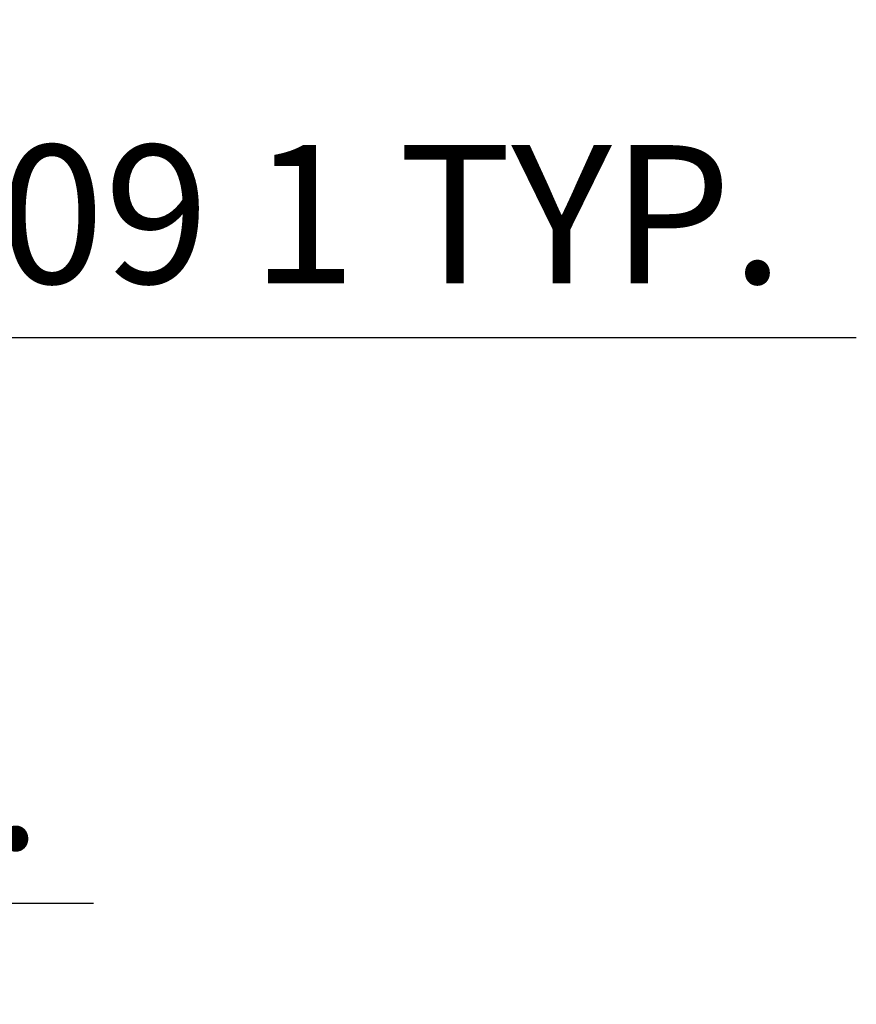
# Model space of a CAD drawing. Units: metres. Extents: x 1246 to 2549, y 2050 to 4184.
# Tile 5 of 6: x 1297 to 1312, y 2088 to 2106. Entities that reach past the tile are written whole.
import ezdxf

# ---------------------------------------------------------------- set-up
doc = ezdxf.new("R2010")
doc.units = ezdxf.units.M
doc.layers.add('A-ANNO-DIMS', color=2, linetype='Continuous', lineweight=18)
doc.styles.get("Standard").update_dxf_attribs({"font": 'arial.ttf'})
doc.dimstyles.new('ISO-25', dxfattribs={"dimtxt": 2.5, "dimasz": 2.5, "dimexe": 1.25, "dimexo": 0.625, "dimtad": 1, "dimtxsty": 'Standard', "dimcen": 2.5, "dimadec": 0, "dimazin": 0, "dimtfac": 1, "dimtmove": 0, "dimatfit": 3, "dimfxl": 1, "dimarcsym": 0})

# ---------------------------------------------------------------- blocks, each defined once
blk = doc.blocks.new('*D10')
at = {"layer": 'A-ANNO-DIMS', "color": 0, "lineweight": -2, "transparency": 16777216}
for p, q in [((1279.137, 2090.073), (1276.637, 2090.073)), ((1281.637, 2090.073), (1281.867, 2090.073)), ((1284.367, 2090.073), (1298.343, 2090.073)), ((1281.637, 2089.585), (1281.637, 2088.823)), ((1281.867, 2089.585), (1281.867, 2088.823))]:
    blk.add_line(p, q, dxfattribs=at)
at = {"layer": 'A-ANNO-DIMS', "color": 0, "transparency": 16777216}
for points in [[(1279.137, 2090.489), (1279.137, 2089.656), (1281.637, 2090.073)], [(1284.367, 2090.489), (1284.367, 2089.656), (1281.867, 2090.073)]]:
    blk.add_solid(points, dxfattribs=at)
at = {"layer": 'Defpoints', "color": 0, "transparency": 16777216}
for p in [(1281.637, 2090.21), (1281.867, 2090.21), (1281.867, 2090.073)]:
    blk.add_point(p, dxfattribs=at)
at = {"layer": 'A-ANNO-DIMS', "color": 0, "transparency": 16777216, "insert": (1292.605, 2091.974), "char_height": 2.5, "attachment_point": 5}
blk.add_mtext('0 TYP.', dxfattribs=at)
blk = doc.blocks.new('*D11')
at = {"layer": 'A-ANNO-DIMS', "color": 0, "lineweight": -2, "transparency": 16777216}
for p, q in [((1280.187, 2100.832), (1280.187, 2101.548)), ((1280.797, 2100.832), (1280.797, 2101.548)), ((1277.687, 2100.298), (1275.187, 2100.298)), ((1280.187, 2100.298), (1280.797, 2100.298)), ((1283.297, 2100.298), (1312.125, 2100.298))]:
    blk.add_line(p, q, dxfattribs=at)
at = {"layer": 'A-ANNO-DIMS', "color": 0, "transparency": 16777216}
for points in [[(1277.687, 2100.715), (1277.687, 2099.882), (1280.187, 2100.298)], [(1283.297, 2100.715), (1283.297, 2099.882), (1280.797, 2100.298)]]:
    blk.add_solid(points, dxfattribs=at)
at = {"layer": 'Defpoints', "color": 0, "transparency": 16777216}
for p in [(1280.797, 2100.298), (1280.187, 2100.207), (1280.797, 2100.207)]:
    blk.add_point(p, dxfattribs=at)
at = {"layer": 'A-ANNO-DIMS', "color": 0, "transparency": 16777216, "insert": (1298.961, 2102.2), "char_height": 2.5, "attachment_point": 5}
blk.add_mtext('WIN-609 1 TYP.', dxfattribs=at)

msp = doc.modelspace()

# ---------------------------------------------------------------- dimensions: what is measured, and where the dimension line sits
at = {"layer": 'A-ANNO-DIMS'}
for base, p1, p2, text, picture, middle in [((1280.7965, 2100.2985), (1280.1873, 2100.2071), (1280.7965, 2100.2071), 'WIN-609 <> TYP.', '*D11', (1298.9607, 2102.1999)), ((1281.8666, 2090.0728), (1281.6366, 2090.2099), (1281.8666, 2090.2099), '<> TYP.', '*D10', (1292.605, 2091.9742))]:
    dim = msp.add_linear_dim(base=base, p1=p1, p2=p2, text=text, dimstyle='ISO-25', override={"dimdec": 0, "dimlfac": 1, "dimrnd": 0, "dimzin": 0, "dimdsep": 46, "dimlunit": 2}, dxfattribs=at)
    dim.commit()
    dim.dimension.update_dxf_attribs({"geometry": picture, "text_midpoint": middle})

doc.saveas('drawing.dxf')
